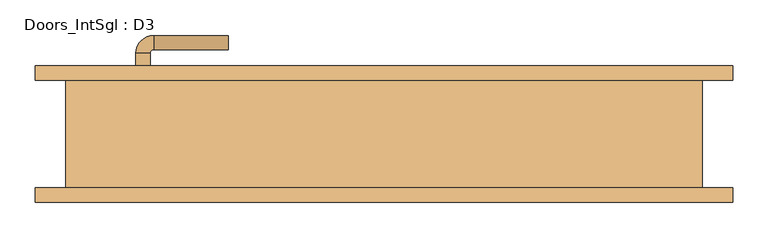
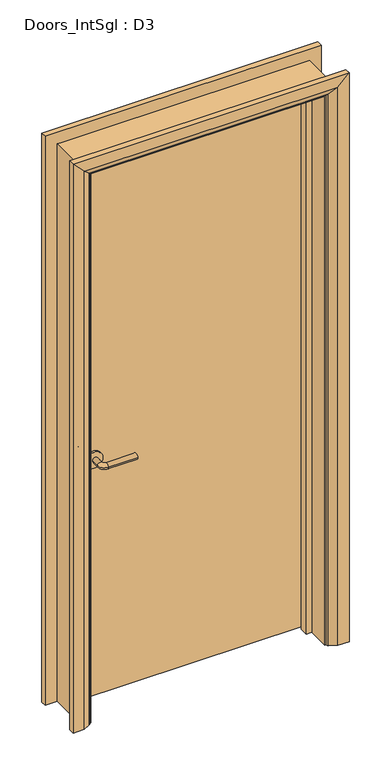
"""IFC4 building model written with IfcOpenShell, lengths in millimetres: door geometry, Doors_IntSgl : D3."""

from ifc_helpers import new_model, si_unit, point, frame, frame_2d, origin, place, context, project, spatial, polyline, circle_curve, ellipse_curve, trimmed, segment, composite_curve, outline, extrude, faceted_brep, source, transform, mapped, element, save
from ifc_brep_helpers import plane_surface, cylinder_surface, revolved_surface, advanced_brep


def doors_intsgl_d3_6b78dd6f(model_context):
    return source(origin(), model_context, "Body", "SolidModel", [
        advanced_brep(
        [(-350.2, 30.2, 900.0), (-330.2, 30.2, 900.0), (-330.2, 0.2, 900.0), (-350.2, 0.2, 900.0), (-325.2, -4.8, 900.0), (-325.2, -24.8, 900.0), (-220.2, -24.8, 900.0), (-220.2, -4.8, 900.0)],
        [
            (0, 1, circle_curve(frame((-340.2, 30.2, 900.0), z_axis=(0.0, 1.0, 0.0), x_axis=(1.0, 0.0, 0.0)), 10.0)),
            (1, 0, circle_curve(frame((-340.2, 30.2, 900.0), z_axis=(0.0, 1.0, 0.0), x_axis=(1.0, 0.0, 0.0)), 10.0)),
            (1, 2),
            (2, 3, circle_curve(frame((-340.2, 0.2, 900.0), z_axis=(0.0, 1.0, 0.0), x_axis=(1.0, 0.0, 0.0)), 10.0)),
            (3, 0),
            (3, 2, circle_curve(frame((-340.2, 0.2, 900.0), z_axis=(0.0, 1.0, 0.0), x_axis=(1.0, 0.0, 0.0)), 10.0)),
            (4, 5, circle_curve(frame((-325.2, -14.8, 900.0), z_axis=(-1.0, 0.0, 0.0), x_axis=(0.0, 1.0, 0.0)), 10.0)),
            (5, 3, circle_curve(frame((-325.2, 0.2, 900.0), z_axis=(0.0, 0.0, -1.0), x_axis=(-1.0, 0.0, 0.0)), 25.0)),
            (2, 4, circle_curve(frame((-325.2, 0.2, 900.0), z_axis=(0.0, 0.0, 1.0), x_axis=(-1.0, 0.0, 0.0)), 5.0)),
            (5, 4, circle_curve(frame((-325.2, -14.8, 900.0), z_axis=(-1.0, 0.0, 0.0), x_axis=(0.0, 1.0, 0.0)), 10.0)),
            (6, 7, circle_curve(frame((-220.2, -14.8, 900.0), z_axis=(1.0, 0.0, 0.0), x_axis=(0.0, 1.0, 0.0)), 10.0)),
            (7, 6, circle_curve(frame((-220.2, -14.8, 900.0), z_axis=(1.0, 0.0, 0.0), x_axis=(0.0, 1.0, 0.0)), 10.0)),
            (4, 7),
            (6, 5),
        ],
        [
            plane_surface(frame((-340.2, 30.2, 900.0), z_axis=(0.0, 1.0, 0.0), x_axis=(0.0, 0.0, 1.0))),
            cylinder_surface(frame((-340.2, 30.2, 900.0), z_axis=(0.0, 1.0, 0.0), x_axis=(1.0, 0.0, 0.0)), 10.0),
            revolved_surface(trimmed(ellipse_curve(frame((-340.2, 0.2, 900.0), z_axis=(0.0, -1.0, 0.0), x_axis=(1.0, 0.0, 0.0)), 10.0, 10.0), [point((-350.2, 0.2, 900.0))], [point((-330.2, 0.2, 900.0))], True, "CARTESIAN"), (-325.2, 0.2, 900.0), (0.0, 0.0, -1.0)),
            revolved_surface(trimmed(ellipse_curve(frame((-340.2, 0.2, 900.0), z_axis=(0.0, -1.0, 0.0), x_axis=(1.0, 0.0, 0.0)), 10.0, 10.0), [point((-330.2, 0.2, 900.0))], [point((-350.2, 0.2, 900.0))], True, "CARTESIAN"), (-325.2, 0.2, 900.0), (0.0, 0.0, -1.0)),
            plane_surface(frame((-220.2, -14.8, 900.0), z_axis=(1.0, 0.0, 0.0), x_axis=(0.0, 0.0, 1.0))),
            cylinder_surface(frame((-325.2, -14.8, 900.0), z_axis=(-1.0, 0.0, 0.0), x_axis=(0.0, 1.0, 0.0)), 10.0),
        ],
        [
            (0, [[1, 2]]),
            (1, [[3, 4, 5, -2]]),
            (1, [[-5, 6, -3, -1]]),
            (2, [[7, 8, -4, 9]]),
            (3, [[10, -9, -6, -8]]),
            (4, [[11, 12]]),
            (5, [[13, -11, 14, -7]]),
            (5, [[-14, -12, -13, -10]]),
        ],
    ),
        extrude(outline(composite_curve([segment(trimmed(circle_curve(frame_2d((900.0, -342.7)), 30.0), [point((900.0, -372.7))], [point((900.0, -312.7))], False, "CARTESIAN"), True, "CONTINUOUS"), segment(trimmed(circle_curve(frame_2d((900.0, -342.7)), 30.0), [point((900.0, -312.7))], [point((900.0, -372.7))], False, "CARTESIAN"), True, "CONTINUOUS")], self_intersect=False)), frame((0.0, 30.2, 0.0), z_axis=(0.0, 1.0, 0.0), x_axis=(0.0, 0.0, 1.0)), (0.0, 0.0, 1.0), 8.0),
        advanced_brep(
        [(-350.2, 84.2, 900.0), (-330.2, 84.2, 900.0), (-350.2, 114.2, 900.0), (-330.2, 114.2, 900.0), (-325.2, 119.2, 900.0), (-325.2, 139.2, 900.0), (-220.2, 139.2, 900.0), (-220.2, 119.2, 900.0)],
        [
            (0, 1, circle_curve(frame((-340.2, 84.2, 900.0), z_axis=(0.0, -1.0, 0.0), x_axis=(1.0, 0.0, 0.0)), 10.0)),
            (1, 0, circle_curve(frame((-340.2, 84.2, 900.0), z_axis=(0.0, -1.0, 0.0), x_axis=(1.0, 0.0, 0.0)), 10.0)),
            (0, 2),
            (2, 3, circle_curve(frame((-340.2, 114.2, 900.0), z_axis=(0.0, -1.0, 0.0), x_axis=(1.0, 0.0, 0.0)), 10.0)),
            (3, 1),
            (3, 2, circle_curve(frame((-340.2, 114.2, 900.0), z_axis=(0.0, -1.0, 0.0), x_axis=(1.0, 0.0, 0.0)), 10.0)),
            (4, 3, circle_curve(frame((-325.2, 114.2, 900.0), z_axis=(0.0, 0.0, 1.0), x_axis=(-1.0, 0.0, 0.0)), 5.0)),
            (2, 5, circle_curve(frame((-325.2, 114.2, 900.0), z_axis=(0.0, 0.0, -1.0), x_axis=(-1.0, 0.0, 0.0)), 25.0)),
            (5, 4, circle_curve(frame((-325.2, 129.2, 900.0), z_axis=(-1.0, 0.0, 0.0), x_axis=(0.0, -1.0, 0.0)), 10.0)),
            (4, 5, circle_curve(frame((-325.2, 129.2, 900.0), z_axis=(-1.0, 0.0, 0.0), x_axis=(0.0, -1.0, 0.0)), 10.0)),
            (6, 7, circle_curve(frame((-220.2, 129.2, 900.0), z_axis=(1.0, 0.0, 0.0), x_axis=(0.0, -1.0, 0.0)), 10.0)),
            (7, 6, circle_curve(frame((-220.2, 129.2, 900.0), z_axis=(1.0, 0.0, 0.0), x_axis=(0.0, -1.0, 0.0)), 10.0)),
            (5, 6),
            (7, 4),
        ],
        [
            plane_surface(frame((-340.2, 84.2, 900.0), z_axis=(0.0, -1.0, 0.0), x_axis=(0.0, 0.0, 1.0))),
            cylinder_surface(frame((-340.2, 84.2, 900.0), z_axis=(0.0, -1.0, 0.0), x_axis=(1.0, 0.0, 0.0)), 10.0),
            revolved_surface(trimmed(ellipse_curve(frame((-340.2, 114.2, 900.0), z_axis=(0.0, -1.0, 0.0), x_axis=(1.0, 0.0, 0.0)), 10.0, 10.0), [point((-350.2, 114.2, 900.0))], [point((-330.2, 114.2, 900.0))], True, "CARTESIAN"), (-325.2, 114.2, 900.0), (0.0, 0.0, -1.0)),
            revolved_surface(trimmed(ellipse_curve(frame((-340.2, 114.2, 900.0), z_axis=(0.0, -1.0, 0.0), x_axis=(1.0, 0.0, 0.0)), 10.0, 10.0), [point((-330.2, 114.2, 900.0))], [point((-350.2, 114.2, 900.0))], True, "CARTESIAN"), (-325.2, 114.2, 900.0), (0.0, 0.0, -1.0)),
            plane_surface(frame((-220.2, 129.2, 900.0), z_axis=(1.0, 0.0, 0.0), x_axis=(0.0, 0.0, 1.0))),
            cylinder_surface(frame((-325.2, 129.2, 900.0), z_axis=(-1.0, 0.0, 0.0), x_axis=(0.0, -1.0, 0.0)), 10.0),
        ],
        [
            (0, [[1, 2]]),
            (1, [[-1, 3, 4, 5]]),
            (1, [[-2, -5, 6, -3]]),
            (2, [[7, -4, 8, 9]]),
            (3, [[-8, -6, -7, 10]]),
            (4, [[11, 12]]),
            (5, [[-9, 13, -12, 14]]),
            (5, [[-10, -14, -11, -13]]),
        ],
    ),
        extrude(outline(composite_curve([segment(trimmed(circle_curve(frame_2d((900.0, -342.7)), 30.0), [point((900.0, -372.7))], [point((900.0, -312.7))], False, "CARTESIAN"), True, "CONTINUOUS"), segment(trimmed(circle_curve(frame_2d((900.0, -342.7)), 30.0), [point((900.0, -312.7))], [point((900.0, -372.7))], False, "CARTESIAN"), True, "CONTINUOUS")], self_intersect=False)), frame((0.0, 76.2, 0.0), z_axis=(0.0, 1.0, 0.0), x_axis=(0.0, 0.0, 1.0)), (0.0, 0.0, 1.0), 8.0),
        extrude(outline(polyline([(415.2, 38.2), (-415.2, 38.2), (-415.2, 76.2), (415.2, 76.2), (415.2, 38.2)])), frame((0.0, 0.0, 8.0), z_axis=(0.0, 0.0, 1.0), x_axis=(1.0, 0.0, 0.0)), (0.0, 0.0, 1.0), 2060.0),
        advanced_brep(
        [(492.2, 96.2, 0.0), (492.2, 76.2, 0.0), (422.2, 76.2, 0.0), (426.2, 82.2, 0.0), (452.2, 96.2, 0.0), (492.2, 96.2, 2145.0), (492.2, 76.2, 2145.0), (-492.2, 76.2, 2145.0), (-492.2, 76.2, 0.0), (-422.2, 76.2, 0.0), (-422.2, 76.2, 2075.0), (422.2, 76.2, 2075.0), (426.2, 82.2, 2079.0), (452.2, 96.2, 2105.0), (-452.2, 96.2, 2105.0), (-452.2, 96.2, 0.0), (-492.2, 96.2, 0.0), (-492.2, 96.2, 2145.0), (-426.2, 82.2, 0.0), (-426.2, 82.2, 2079.0)],
        [
            (0, 1),
            (1, 2),
            (2, 3, circle_curve(frame((430.2, 75.2, 0.0), z_axis=(0.0, 0.0, -1.0), x_axis=(1.0, 0.0, 0.0)), 8.0622577)),
            (3, 4),
            (4, 0),
            (0, 5),
            (5, 6),
            (6, 1),
            (6, 7),
            (7, 8),
            (8, 9),
            (9, 10),
            (10, 11),
            (11, 2),
            (11, 12, ellipse_curve(frame((430.2, 75.2, 2083.0), z_axis=(0.7071067811865475, 0.0, -0.7071067811865475), x_axis=(-0.7071067811865474, 0.0, -0.7071067811865476)), 11.4017543, 8.0622577)),
            (12, 3),
            (12, 13),
            (13, 4),
            (13, 14),
            (14, 15),
            (15, 16),
            (16, 17),
            (17, 5),
            (7, 17),
            (16, 8),
            (15, 18),
            (18, 9, circle_curve(frame((-430.2, 75.2, 0.0), z_axis=(0.0, 0.0, -1.0), x_axis=(-1.0, 0.0, 0.0)), 8.0622577)),
            (19, 10, ellipse_curve(frame((-430.2, 75.2, 2083.0), z_axis=(-0.7071067811865475, 0.0, -0.7071067811865475), x_axis=(-0.7071067811865474, 0.0, 0.7071067811865476)), 11.4017543, 8.0622577)),
            (18, 19),
            (14, 19),
            (19, 12),
        ],
        [
            plane_surface(frame((422.2, 76.2, 0.0), z_axis=(0.0, 0.0, -1.0), x_axis=(0.0, -1.0, 0.0))),
            plane_surface(frame((492.2, 96.2, 0.0), z_axis=(1.0, 0.0, 0.0), x_axis=(0.0, 0.0, 1.0))),
            plane_surface(frame((492.2, 76.2, 0.0), z_axis=(0.0, -1.0, 0.0), x_axis=(0.0, 0.0, 1.0))),
            cylinder_surface(frame((430.2, 75.2, 0.0), z_axis=(0.0, 0.0, -1.0), x_axis=(1.0, 0.0, 0.0)), 8.0622577),
            plane_surface(frame((426.2, 82.2, 0.0), z_axis=(-0.4740998230350126, 0.880471099922178, 0.0), x_axis=(0.0, 0.0, 1.0))),
            plane_surface(frame((452.2, 96.2, 0.0), z_axis=(0.0, 1.0, 0.0), x_axis=(0.0, 0.0, 1.0))),
            plane_surface(frame((-492.2, 96.2, 2145.0), z_axis=(-1.0, 0.0, 0.0), x_axis=(0.0, 0.0, -1.0))),
            plane_surface(frame((-422.2, 76.2, 0.0), z_axis=(0.0, 0.0, -1.0), x_axis=(0.0, -1.0, 0.0))),
            cylinder_surface(frame((-430.2, 75.2, 2075.0), z_axis=(0.0, 0.0, 1.0), x_axis=(-1.0, 0.0, 0.0)), 8.0622577),
            plane_surface(frame((-426.2, 82.2, 2079.0), z_axis=(0.47409982303501824, 0.8804710999221749, 0.0), x_axis=(0.0, 0.0, -1.0))),
            plane_surface(frame((492.2, 96.2, 2145.0), z_axis=(0.0, 0.0, 1.0), x_axis=(-1.0, 0.0, 0.0))),
            cylinder_surface(frame((422.2, 75.2, 2083.0), z_axis=(1.0, 0.0, 0.0), x_axis=(0.0, 0.0, 1.0)), 8.0622577),
            plane_surface(frame((426.2, 82.2, 2079.0), z_axis=(0.0, 0.8804710999221764, -0.4740998230350154), x_axis=(-1.0, 0.0, 0.0))),
        ],
        [
            (0, [[1, 2, 3, 4, 5]]),
            (1, [[-1, 6, 7, 8]]),
            (2, [[-2, -8, 9, 10, 11, 12, 13, 14]]),
            (3, [[-3, -14, 15, 16]]),
            (4, [[-4, -16, 17, 18]]),
            (5, [[-5, -18, 19, 20, 21, 22, 23, -6]]),
            (6, [[24, -22, 25, -10]]),
            (7, [[-21, 26, 27, -11, -25]]),
            (8, [[28, -12, -27, 29]]),
            (9, [[30, -29, -26, -20]]),
            (10, [[-7, -23, -24, -9]]),
            (11, [[-15, -13, -28, 31]]),
            (12, [[-17, -31, -30, -19]]),
        ],
    ),
        extrude(outline(polyline([(0.0, -417.2), (0.0, -398.2), (2051.0, -398.2), (2051.0, 398.2), (0.0, 398.2), (0.0, 417.2), (2070.0, 417.2), (2070.0, -417.2), (0.0, -417.2)])), frame((0.0, 4.2, 0.0), z_axis=(0.0, 1.0, 0.0), x_axis=(0.0, 0.0, 1.0)), (0.0, 0.0, 1.0), 32.0),
        advanced_brep(
        [(-492.2, -96.2, 0.0), (-492.2, -76.2, 0.0), (-422.2, -76.2, 0.0), (-426.2, -82.2, 0.0), (-452.2, -96.2, 0.0), (-492.2, -96.2, 2145.0), (-492.2, -76.2, 2145.0), (-422.2, -76.2, 2075.0), (-426.2, -82.2, 2079.0), (-452.2, -96.2, 2105.0), (492.2, -96.2, 0.0), (452.2, -96.2, 0.0), (426.2, -82.2, 0.0), (422.2, -76.2, 0.0), (492.2, -76.2, 0.0), (492.2, -96.2, 2145.0), (452.2, -96.2, 2105.0), (426.2, -82.2, 2079.0), (422.2, -76.2, 2075.0), (492.2, -76.2, 2145.0)],
        [
            (0, 1),
            (1, 2),
            (2, 3, circle_curve(frame((-430.2, -75.2, 0.0), z_axis=(0.0, 0.0, -1.0), x_axis=(-1.0, 0.0, 0.0)), 8.0622577)),
            (3, 4),
            (4, 0),
            (0, 5),
            (5, 6),
            (6, 1),
            (6, 7),
            (7, 2),
            (7, 8, ellipse_curve(frame((-430.2, -75.2, 2083.0), z_axis=(-0.7071067811865475, 0.0, -0.7071067811865475), x_axis=(0.7071067811865474, 0.0, -0.7071067811865476)), 11.4017543, 8.0622577)),
            (8, 3),
            (8, 9),
            (9, 4),
            (9, 5),
            (10, 11),
            (11, 12),
            (12, 13, circle_curve(frame((430.2, -75.2, 0.0), z_axis=(0.0, 0.0, -1.0), x_axis=(1.0, 0.0, 0.0)), 8.0622577)),
            (13, 14),
            (14, 10),
            (15, 16),
            (16, 11),
            (10, 15),
            (16, 17),
            (17, 12),
            (17, 18, ellipse_curve(frame((430.2, -75.2, 2083.0), z_axis=(0.7071067811865475, 0.0, -0.7071067811865475), x_axis=(0.7071067811865474, 0.0, 0.7071067811865476)), 11.4017543, 8.0622577)),
            (18, 13),
            (18, 19),
            (19, 14),
            (19, 15),
            (5, 15),
            (19, 6),
            (18, 7),
            (17, 8),
            (16, 9),
        ],
        [
            plane_surface(frame((-422.2, -149.0010989, 0.0), z_axis=(0.0, 0.0, -1.0), x_axis=(1.0, 0.0, 0.0))),
            plane_surface(frame((-492.2, -96.2, 0.0), z_axis=(-1.0, 0.0, 0.0), x_axis=(0.0, 0.0, 1.0))),
            plane_surface(frame((-492.2, -76.2, 0.0), z_axis=(0.0, 1.0, 0.0), x_axis=(0.0, 0.0, 1.0))),
            cylinder_surface(frame((-430.2, -75.2, 0.0), z_axis=(0.0, 0.0, -1.0), x_axis=(-1.0, 0.0, 0.0)), 8.0622577),
            plane_surface(frame((-426.2, -82.2, 0.0), z_axis=(0.4740998230350183, -0.8804710999221749, 0.0), x_axis=(0.0, 0.0, 1.0))),
            plane_surface(frame((-452.2, -96.2, 0.0), z_axis=(0.0, -1.0, 0.0), x_axis=(0.0, 0.0, 1.0))),
            plane_surface(frame((422.2, -149.0010989, 0.0), z_axis=(0.0, 0.0, -1.0), x_axis=(-1.0, 0.0, 0.0))),
            plane_surface(frame((452.2, -96.2, 2105.0), z_axis=(0.0, -1.0, 0.0), x_axis=(0.0, 0.0, -1.0))),
            plane_surface(frame((426.2, -82.2, 2079.0), z_axis=(-0.4740998230350183, -0.8804710999221749, 0.0), x_axis=(0.0, 0.0, -1.0))),
            cylinder_surface(frame((430.2, -75.2, 2075.0), z_axis=(0.0, 0.0, 1.0), x_axis=(1.0, 0.0, 0.0)), 8.0622577),
            plane_surface(frame((492.2, -76.2, 2145.0), z_axis=(0.0, 1.0, 0.0), x_axis=(0.0, 0.0, -1.0))),
            plane_surface(frame((492.2, -96.2, 2145.0), z_axis=(1.0, 0.0, 0.0), x_axis=(0.0, 0.0, -1.0))),
            plane_surface(frame((-492.2, -96.2, 2145.0), z_axis=(0.0, 0.0, 1.0), x_axis=(1.0, 0.0, 0.0))),
            plane_surface(frame((-492.2, -76.2, 2145.0), z_axis=(0.0, 1.0, 0.0), x_axis=(1.0, 0.0, 0.0))),
            cylinder_surface(frame((-422.2, -75.2, 2083.0), z_axis=(-1.0, 0.0, 0.0), x_axis=(0.0, 0.0, 1.0)), 8.0622577),
            plane_surface(frame((-426.2, -82.2, 2079.0), z_axis=(0.0, -0.8804710999221749, -0.4740998230350183), x_axis=(1.0, 0.0, 0.0))),
            plane_surface(frame((-452.2, -96.2, 2105.0), z_axis=(0.0, -1.0, 0.0), x_axis=(1.0, 0.0, 0.0))),
        ],
        [
            (0, [[1, 2, 3, 4, 5]]),
            (1, [[-1, 6, 7, 8]]),
            (2, [[-2, -8, 9, 10]]),
            (3, [[-3, -10, 11, 12]]),
            (4, [[-4, -12, 13, 14]]),
            (5, [[-5, -14, 15, -6]]),
            (6, [[16, 17, 18, 19, 20]]),
            (7, [[21, 22, -16, 23]]),
            (8, [[24, 25, -17, -22]]),
            (9, [[26, 27, -18, -25]]),
            (10, [[28, 29, -19, -27]]),
            (11, [[30, -23, -20, -29]]),
            (12, [[-7, 31, -30, 32]]),
            (13, [[-9, -32, -28, 33]]),
            (14, [[-11, -33, -26, 34]]),
            (15, [[-13, -34, -24, 35]]),
            (16, [[-15, -35, -21, -31]]),
        ],
    ),
        faceted_brep([(-417.2, 76.2, 0.0), (-417.2, -76.2, 0.0), (-449.2, -76.2, 0.0), (-449.2, 76.2, 0.0), (-417.2, 76.2, 2070.0), (-417.2, -76.2, 2070.0), (-449.2, -76.2, 2102.0), (-449.2, 76.2, 2102.0), (417.2, 76.2, 0.0), (449.2, 76.2, 0.0), (449.2, -76.2, 0.0), (417.2, -76.2, 0.0), (417.2, 76.2, 2070.0), (449.2, 76.2, 2102.0), (449.2, -76.2, 2102.0), (417.2, -76.2, 2070.0)], [[[0, 1, 2, 3]], [[1, 0, 4, 5]], [[2, 1, 5, 6]], [[3, 2, 6, 7]], [[0, 3, 7, 4]], [[8, 9, 10, 11]], [[12, 13, 9, 8]], [[13, 14, 10, 9]], [[14, 15, 11, 10]], [[15, 12, 8, 11]], [[5, 4, 12, 15]], [[6, 5, 15, 14]], [[7, 6, 14, 13]], [[4, 7, 13, 12]]]),
    ])


if __name__ == "__main__":
    model = new_model("IFC4")
    model_context = context("Model", 3, world=origin())
    ifc_project = project(units=[si_unit("LENGTHUNIT", "METRE", prefix="MILLI")], contexts=[model_context])
    site = spatial("IfcSite", under=ifc_project)
    building = spatial("IfcBuilding", under=site)
    placement = place(None, origin())
    doors_intsgl_d3_shape = doors_intsgl_d3_6b78dd6f(model_context)
    element("IfcDoor", 1, ObjectType="Doors_IntSgl : D3", at=placement, inside=building, context=model_context, shape_type="MappedRepresentation", body=[
        mapped(doors_intsgl_d3_shape, transform((0.0, 0.0, 0.0), x_axis=(1.0, 0.0, 0.0), y_axis=(0.0, 1.0, 0.0), z_axis=(0.0, 0.0, 1.0))),
    ])
    save(model, "model.ifc")

# Revit data of these elements
# Type "Doors_IntSgl : D3"
#   Type Mark = "51"
#   Type Comments = "Internal Single"
#   Operation = "SingleSwingRight"
#   Manufacturer = "Revit"
#   Keynote = "L20"
#   Description = "Internal Single Door"
#   Analytic Construction = "Metal"
#   UnderCut = 0.026247 ft
#   Tolerance = 0.006562 ft
#   Thickness = 0.124672 ft
#   Thermal Resistance (R) = 0.270117 (m²·K)/W
#   Structural Tolerance = 0.026247 ft
#   StopDepth = 0.104987 ft
#   Stop Thickness = 0.062336 ft
#   Rough Width = 3.0 ft
#   Rough Height = 6.922572 ft
#   Height to Top Lock Rail = 3.28084 ft
#   Heat Transfer Coefficient (U) = 3.7021 W/(m²·K)
#   Handle Z Distance = 2.952756 ft
#   Handle X Distance = 0.246063 ft
#   Frame Thickness = 0.104987 ft
#   Door Panel Width = 2.724409 ft
#   Door Panel Thickness = 0.124672 ft
#   Door Panel Offset = 0.0 ft
#   Height = 6.922572 ft
#   Width = 3.0 ft
#   Door Panel Height = 6.75853 ft
#   Architrave Setback = 0.016404 ft
#   Vis - Ironmongery = yes
#   Material Ironmongery = Door - Handle
#   Material Frame = Door - Frame/Mullion (1)
#   Material Door = Door - Panel
#   Material Architrave = Door - Architrave
#   Visual Light Transmittance = 0
#   Solar Heat Gain Coefficient = 0
#   Function = (empty or 0)
#   Wall Closure = (empty or 0)
# Element 1 (IfcDoor, "Doors_IntSgl : D3")
#   Materials on its faces: "Door - Architrave", "Door - Handle", "Door - Frame/Mullion (1)", "Door - Panel"
# Materials
#   "Door - Handle": colour RGB 0 0 0, transparency 0, Keynote = "P21", Cost = 0
#   "Door - Frame/Mullion (1)": class "Wood", colour RGB 212 179 113, transparency 0, Keynote = "L20", Cost = 0
#   "Door - Panel": class "Wood", colour RGB 210 159 95, transparency 0, Keynote = "L20", Cost = 0
#   "Door - Architrave": class "Wood", colour RGB 154 90 5, transparency 0, Keynote = "P20", Cost = 0
